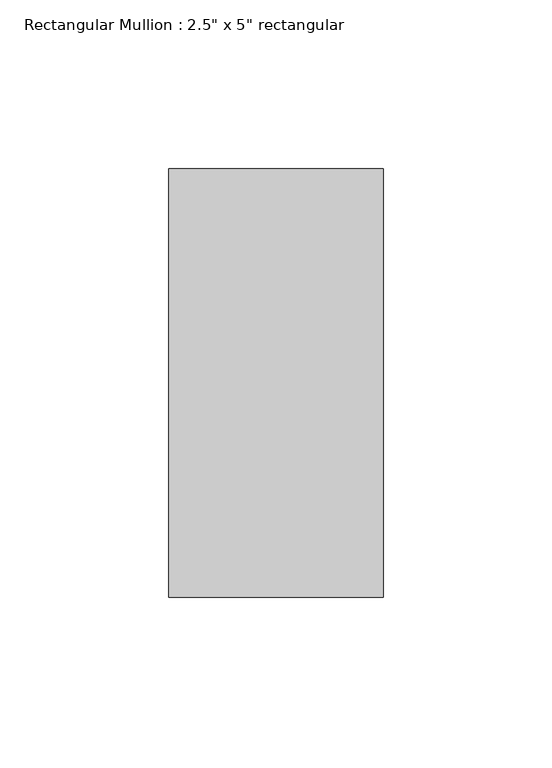
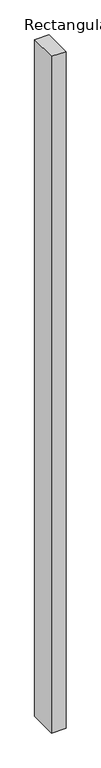
"""IFC4 building model written with IfcOpenShell, lengths in millimetres: member geometry."""

from ifc_helpers import new_model, si_unit, frame, origin, place, context, project, spatial, polyline, outline, extrude, source, transform, mapped, element, save


def member_e3dca2c5(model_context):
    return source(origin(), model_context, "Body", "SweptSolid", [
        extrude(outline(polyline([(0.0, 63.5), (0.0, -63.5), (-63.5, -63.5), (-63.5, 63.5), (0.0, 63.5)])), frame((0.0, 0.0, -3116.4241767), z_axis=(0.0, 0.0, 1.0), x_axis=(1.0, 0.0, 0.0)), (0.0, 0.0, 1.0), 3116.4241767),
    ])


if __name__ == "__main__":
    model = new_model("IFC4")
    model_context = context("Model", 3, world=origin())
    ifc_project = project(units=[si_unit("LENGTHUNIT", "METRE", prefix="MILLI")], contexts=[model_context])
    site = spatial("IfcSite", under=ifc_project)
    building = spatial("IfcBuilding", under=site)
    placement = place(None, origin())
    member_shape = member_e3dca2c5(model_context)
    element("IfcMember", 1, ObjectType="Rectangular Mullion : 2.5\" x 5\" rectangular", at=placement, inside=building, context=model_context, shape_type="MappedRepresentation", body=[
        mapped(member_shape, transform((0.0, 0.0, 0.0), x_axis=(1.0, 0.0, 0.0), y_axis=(0.0, 1.0, 0.0), z_axis=(0.0, 0.0, 1.0))),
    ])
    save(model, "model.ifc")

# Revit data of these elements
# Type "Rectangular Mullion : 2.5\" x 5\" rectangular"
#   built-in parameter 1007304 = 0.416667 (stored number, unit not read)
#   built-in parameter 1007301 = 0.104167 (stored number, unit not read)
#   built-in parameter 1007300 = 0.104167 (stored number, unit not read)
# Element 1 (IfcMember, "Rectangular Mullion : 2.5\" x 5\" rectangular")
#   Materials on its faces: "Aluminum"
# Materials
#   "Aluminum": class "Metal", colour RGB 247 247 247, transparency 0, Description = "Aluminum 6061", Cost = 0
